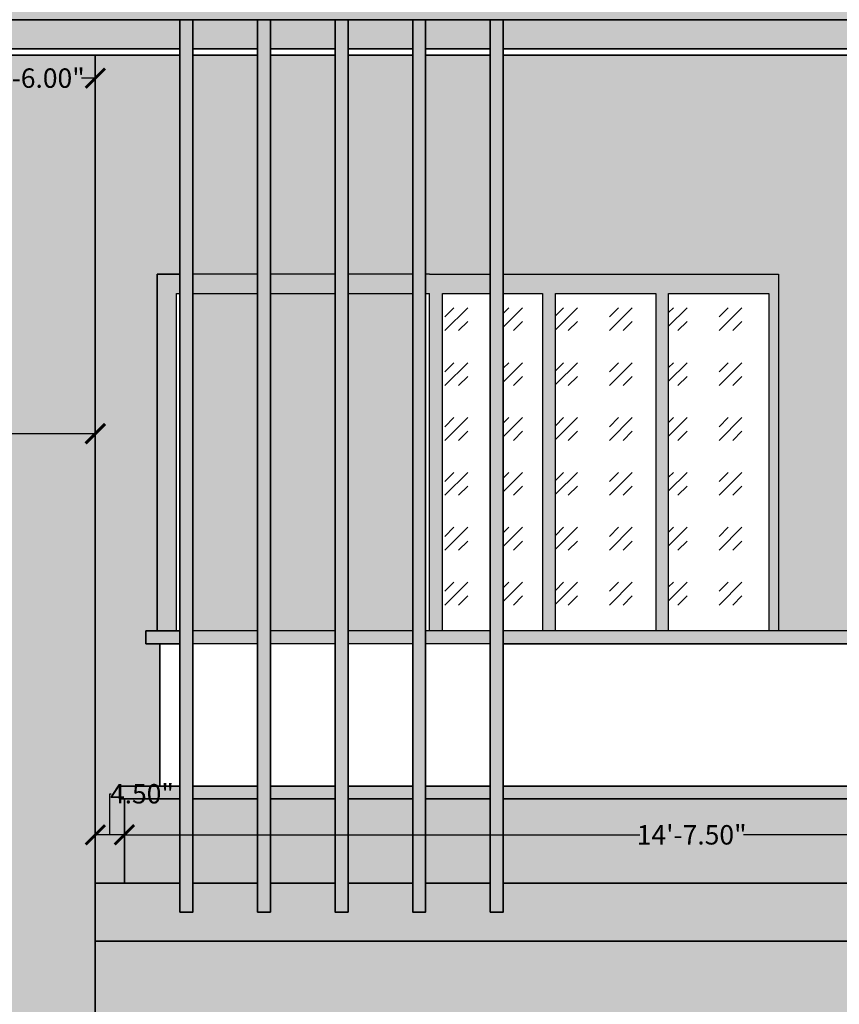
# Model space of a CAD drawing. Units: inches. Extents: x -654 to 390, y -40 to 648.
# Tile 6 of 13: x 104 to 231, y 159 to 311. Entities that reach past the tile are written whole.
import ezdxf

# ---------------------------------------------------------------- set-up
doc = ezdxf.new("R2010")
doc.units = ezdxf.units.IN
doc.header["$PDMODE"] = 3
for name, color, linetype, lineweight in [('A-ANNO-DIMS', 2, 'Continuous', 18), ('A-ELEV', 7, 'Continuous', 35), ('A-ELEV-FILL', 252, 'Continuous', 13), ('A-ELEV-PATT', 8, 'Continuous', 13), ('A-GLAZ', 4, 'Continuous', 25)]:
    doc.layers.add(name, color=color, linetype=linetype, lineweight=lineweight)
doc.styles.get("Standard").update_dxf_attribs({"font": 'arial.ttf'})
doc.dimstyles.get("Standard").update_dxf_attribs({"dimtxt": 3, "dimasz": 3, "dimexe": 0.18, "dimexo": 0.0625, "dimgap": 0.09, "dimtad": 0, "dimtih": 1, "dimtoh": 1, "dimzin": 0, "dimdsep": 46, "dimlunit": 3, "dimtxsty": 'Standard', "dimblk": 'ARCHTICK', "dimcen": 0.09, "dimse1": 1, "dimse2": 1, "dimadec": 0, "dimazin": 0, "dimtfac": 1, "dimtofl": 0, "dimtmove": 0, "dimatfit": 3, "dimfxl": 1, "dimtolj": 1, "dimtzin": 0, "dimarcsym": 0})

# ---------------------------------------------------------------- blocks, each defined once
blk = doc.blocks.new('_ArchTick')
at = {"color": 0, "linetype": 'ByBlock', "const_width": 0.15}
blk.add_lwpolyline([(-0.5, -0.5), (0.5, 0.5)], dxfattribs=at)
blk = doc.blocks.new('*D60')
at = {"layer": 'A-ANNO-DIMS', "color": 0, "lineweight": -2, "transparency": 16777216}
for p, q in [((120.15, 185.09), (199.88, 185.09)), ((295.65, 185.09), (215.91, 185.09))]:
    blk.add_line(p, q, dxfattribs=at)
at = {"layer": 'Defpoints', "color": 0, "transparency": 16777216}
for p in [(120.15, 185.09), (120.15, 185.09), (295.65, 185.09)]:
    blk.add_point(p, dxfattribs=at)
at = {"layer": 'A-ANNO-DIMS', "color": 0, "lineweight": -2, "transparency": 16777216, "xscale": 3, "yscale": 3, "zscale": 3, "rotation": 180}
blk.add_blockref('_ArchTick', (120.15, 185.09), dxfattribs=at)
at = {"layer": 'A-ANNO-DIMS', "color": 0, "lineweight": -2, "transparency": 16777216, "xscale": 3, "yscale": 3, "zscale": 3}
blk.add_blockref('_ArchTick', (295.65, 185.09), dxfattribs=at)
at = {"layer": 'A-ANNO-DIMS', "color": 0, "transparency": 16777216, "insert": (207.9, 185.09), "char_height": 3, "attachment_point": 5}
blk.add_mtext('\\A1;14\'-7.50"', dxfattribs=at)
blk = doc.blocks.new('*D61')
at = {"layer": 'A-ANNO-DIMS', "color": 0, "lineweight": -2, "transparency": 16777216}
for p, q in [((117.9, 185.09), (117.9, 191.44)), ((117.9, 191.44), (118.08, 191.44)), ((120.15, 185.09), (115.65, 185.09))]:
    blk.add_line(p, q, dxfattribs=at)
at = {"layer": 'Defpoints', "color": 0, "transparency": 16777216}
for p in [(115.65, 185.09), (115.65, 185.09), (120.15, 185.09)]:
    blk.add_point(p, dxfattribs=at)
at = {"layer": 'A-ANNO-DIMS', "color": 0, "lineweight": -2, "transparency": 16777216, "xscale": 3, "yscale": 3, "zscale": 3, "rotation": 180}
blk.add_blockref('_ArchTick', (115.65, 185.09), dxfattribs=at)
at = {"layer": 'A-ANNO-DIMS', "color": 0, "lineweight": -2, "transparency": 16777216, "xscale": 3, "yscale": 3, "zscale": 3}
blk.add_blockref('_ArchTick', (120.15, 185.09), dxfattribs=at)
at = {"layer": 'A-ANNO-DIMS', "color": 0, "transparency": 16777216, "insert": (122.86, 191.44), "char_height": 3, "attachment_point": 5}
blk.add_mtext('\\A1;4.50"', dxfattribs=at)
blk = doc.blocks.new('*D69')
at = {"layer": 'A-ANNO-DIMS', "color": 0, "lineweight": -2, "transparency": 16777216}
for p, q in [((57.15, 247.12), (78.18, 247.12)), ((115.65, 247.12), (94.61, 247.12))]:
    blk.add_line(p, q, dxfattribs=at)
at = {"layer": 'Defpoints', "color": 0, "transparency": 16777216}
for p in [(115.65, 247.12), (115.65, 177.63), (57.15, 161.13)]:
    blk.add_point(p, dxfattribs=at)
at = {"layer": 'A-ANNO-DIMS', "color": 0, "lineweight": -2, "transparency": 16777216, "xscale": 3, "yscale": 3, "zscale": 3, "rotation": 180}
blk.add_blockref('_ArchTick', (57.15, 247.12), dxfattribs=at)
at = {"layer": 'A-ANNO-DIMS', "color": 0, "lineweight": -2, "transparency": 16777216, "xscale": 3, "yscale": 3, "zscale": 3}
blk.add_blockref('_ArchTick', (115.65, 247.12), dxfattribs=at)
at = {"layer": 'A-ANNO-DIMS', "color": 0, "transparency": 16777216, "insert": (86.4, 247.12), "char_height": 3, "attachment_point": 5}
blk.add_mtext('\\A1;4\'-10.50"', dxfattribs=at)
blk = doc.blocks.new('*D70')
at = {"layer": 'A-ANNO-DIMS', "color": 0, "lineweight": -2, "transparency": 16777216}
for p, q in [((97.65, 302.1), (99.8, 302.1)), ((115.65, 302.1), (113.5, 302.1))]:
    blk.add_line(p, q, dxfattribs=at)
at = {"layer": 'Defpoints', "color": 0, "transparency": 16777216}
for p in [(97.65, 305.63), (115.65, 305.63), (115.65, 302.1)]:
    blk.add_point(p, dxfattribs=at)
at = {"layer": 'A-ANNO-DIMS', "color": 0, "lineweight": -2, "transparency": 16777216, "xscale": 3, "yscale": 3, "zscale": 3, "rotation": 180}
blk.add_blockref('_ArchTick', (97.65, 302.1), dxfattribs=at)
at = {"layer": 'A-ANNO-DIMS', "color": 0, "lineweight": -2, "transparency": 16777216, "xscale": 3, "yscale": 3, "zscale": 3}
blk.add_blockref('_ArchTick', (115.65, 302.1), dxfattribs=at)
at = {"layer": 'A-ANNO-DIMS', "color": 0, "transparency": 16777216, "insert": (106.65, 302.1), "char_height": 3, "attachment_point": 5}
blk.add_mtext('\\A1;1\'-6.00"', dxfattribs=at)
blk = doc.blocks.new('*D76')
at = {"layer": 'A-ANNO-DIMS', "color": 0, "lineweight": -2, "transparency": 16777216}
for p, q in [((380.75, 611.13), (380.75, 306.76)), ((380.75, -0.87), (380.75, 303.51))]:
    blk.add_line(p, q, dxfattribs=at)
at = {"layer": 'Defpoints', "color": 0, "transparency": 16777216}
for p in [(126.65, 611.13), (380.75, 611.13), (346.65, -0.87)]:
    blk.add_point(p, dxfattribs=at)
at = {"layer": 'A-ANNO-DIMS', "color": 0, "lineweight": -2, "transparency": 16777216, "xscale": 3, "yscale": 3, "zscale": 3}
for p, rotation in [((380.75, 611.13), 90), ((380.75, -0.87), 270)]:
    blk.add_blockref('_ArchTick', p, dxfattribs=dict(at, rotation=rotation))
at = {"layer": 'A-ANNO-DIMS', "color": 0, "transparency": 16777216, "insert": (380.75, 305.13), "char_height": 3, "attachment_point": 5}
blk.add_mtext('\\A1;51\'-0"', dxfattribs=at)
blk = doc.blocks.new('*D92')
at = {"layer": 'A-ANNO-DIMS', "color": 0, "lineweight": -2, "transparency": 16777216}
for p, q in [((115.65, -32.97), (125.23, -32.97)), ((125.23, -32.97), (128.23, -32.97))]:
    blk.add_line(p, q, dxfattribs=at)
at = {"layer": 'Defpoints', "color": 0, "transparency": 16777216}
for p in [(115.65, 305.63), (125.23, 271.79), (125.23, -32.97)]:
    blk.add_point(p, dxfattribs=at)
at = {"layer": 'A-ANNO-DIMS', "color": 0, "lineweight": -2, "transparency": 16777216, "xscale": 3, "yscale": 3, "zscale": 3, "rotation": 180}
blk.add_blockref('_ArchTick', (115.65, -32.97), dxfattribs=at)
at = {"layer": 'A-ANNO-DIMS', "color": 0, "lineweight": -2, "transparency": 16777216, "xscale": 3, "yscale": 3, "zscale": 3}
blk.add_blockref('_ArchTick', (125.23, -32.97), dxfattribs=at)
at = {"layer": 'A-ANNO-DIMS', "color": 0, "transparency": 16777216, "insert": (135.8, -32.97), "char_height": 3, "attachment_point": 5}
blk.add_mtext('\\A1;0\'-9 1/2"', dxfattribs=at)
blk = doc.blocks.new('*D93')
at = {"layer": 'A-ANNO-DIMS', "color": 0, "lineweight": -2, "transparency": 16777216}
for p, q in [((125.23, -32.97), (169.2, -32.97)), ((221.33, -32.97), (177.36, -32.97))]:
    blk.add_line(p, q, dxfattribs=at)
at = {"layer": 'Defpoints', "color": 0, "transparency": 16777216}
for p in [(125.23, 271.79), (221.33, 271.79), (221.33, -32.97)]:
    blk.add_point(p, dxfattribs=at)
at = {"layer": 'A-ANNO-DIMS', "color": 0, "lineweight": -2, "transparency": 16777216, "xscale": 3, "yscale": 3, "zscale": 3, "rotation": 180}
blk.add_blockref('_ArchTick', (125.23, -32.97), dxfattribs=at)
at = {"layer": 'A-ANNO-DIMS', "color": 0, "lineweight": -2, "transparency": 16777216, "xscale": 3, "yscale": 3, "zscale": 3}
blk.add_blockref('_ArchTick', (221.33, -32.97), dxfattribs=at)
at = {"layer": 'A-ANNO-DIMS', "color": 0, "transparency": 16777216, "insert": (173.28, -32.97), "char_height": 3, "attachment_point": 5}
blk.add_mtext('\\A1;8\'-0"', dxfattribs=at)
blk = doc.blocks.new('*D94')
at = {"layer": 'A-ANNO-DIMS', "color": 0, "lineweight": -2, "transparency": 16777216}
for p, q in [((380.75, 271.79), (380.75, 245.8)), ((380.75, 216.63), (380.75, 242.62))]:
    blk.add_line(p, q, dxfattribs=at)
at = {"layer": 'Defpoints', "color": 0, "transparency": 16777216}
for p in [(221.33, 271.79), (244.73, 216.63), (380.75, 216.63)]:
    blk.add_point(p, dxfattribs=at)
at = {"layer": 'A-ANNO-DIMS', "color": 0, "lineweight": -2, "transparency": 16777216, "xscale": 3, "yscale": 3, "zscale": 3}
for p, rotation in [((380.75, 271.79), 90), ((380.75, 216.63), 270)]:
    blk.add_blockref('_ArchTick', p, dxfattribs=dict(at, rotation=rotation))
at = {"layer": 'A-ANNO-DIMS', "color": 0, "transparency": 16777216, "insert": (380.75, 244.21), "char_height": 3, "attachment_point": 5}
blk.add_mtext('\\A1;4\'-7"', dxfattribs=at)
blk = doc.blocks.new('*D97')
at = {"layer": 'A-ANNO-DIMS', "color": 0, "lineweight": -2, "transparency": 16777216}
for p, q in [((128.74, -32.97), (130.81, -32.97)), ((140.74, -32.97), (138.68, -32.97))]:
    blk.add_line(p, q, dxfattribs=at)
at = {"layer": 'Defpoints', "color": 0, "transparency": 16777216}
for p in [(128.74, 173.13), (140.74, 173.13), (140.74, -32.97)]:
    blk.add_point(p, dxfattribs=at)
at = {"layer": 'A-ANNO-DIMS', "color": 0, "lineweight": -2, "transparency": 16777216, "xscale": 3, "yscale": 3, "zscale": 3, "rotation": 180}
blk.add_blockref('_ArchTick', (128.74, -32.97), dxfattribs=at)
at = {"layer": 'A-ANNO-DIMS', "color": 0, "lineweight": -2, "transparency": 16777216, "xscale": 3, "yscale": 3, "zscale": 3}
blk.add_blockref('_ArchTick', (140.74, -32.97), dxfattribs=at)
at = {"layer": 'A-ANNO-DIMS', "color": 0, "transparency": 16777216, "insert": (134.74, -32.97), "char_height": 3, "attachment_point": 5}
blk.add_mtext('\\A1;1\'-0"', dxfattribs=at)
blk = doc.blocks.new('*D98')
at = {"layer": 'A-ANNO-DIMS', "color": 0, "lineweight": -2, "transparency": 16777216}
for p, q in [((128.74, -32.97), (149.6, -32.97)), ((178.74, -32.97), (157.88, -32.97))]:
    blk.add_line(p, q, dxfattribs=at)
at = {"layer": 'Defpoints', "color": 0, "transparency": 16777216}
for p in [(128.74, 173.13), (178.74, 173.13), (178.74, -32.97)]:
    blk.add_point(p, dxfattribs=at)
at = {"layer": 'A-ANNO-DIMS', "color": 0, "lineweight": -2, "transparency": 16777216, "xscale": 3, "yscale": 3, "zscale": 3, "rotation": 180}
blk.add_blockref('_ArchTick', (128.74, -32.97), dxfattribs=at)
at = {"layer": 'A-ANNO-DIMS', "color": 0, "lineweight": -2, "transparency": 16777216, "xscale": 3, "yscale": 3, "zscale": 3}
blk.add_blockref('_ArchTick', (178.74, -32.97), dxfattribs=at)
at = {"layer": 'A-ANNO-DIMS', "color": 0, "transparency": 16777216, "insert": (153.74, -32.97), "char_height": 3, "attachment_point": 5}
blk.add_mtext('\\A1;4\'-2"', dxfattribs=at)
blk = doc.blocks.new('*D99')
at = {"layer": 'A-ANNO-DIMS', "color": 0, "lineweight": -2, "transparency": 16777216}
for p, q in [((380.75, 311.13), (380.75, 243.76)), ((380.75, 173.13), (380.75, 240.51))]:
    blk.add_line(p, q, dxfattribs=at)
at = {"layer": 'Defpoints', "color": 0, "transparency": 16777216}
for p in [(178.74, 311.13), (380.75, 311.13), (178.74, 173.13)]:
    blk.add_point(p, dxfattribs=at)
at = {"layer": 'A-ANNO-DIMS', "color": 0, "lineweight": -2, "transparency": 16777216, "xscale": 3, "yscale": 3, "zscale": 3}
for p, rotation in [((380.75, 311.13), 90), ((380.75, 173.13), 270)]:
    blk.add_blockref('_ArchTick', p, dxfattribs=dict(at, rotation=rotation))
at = {"layer": 'A-ANNO-DIMS', "color": 0, "transparency": 16777216, "insert": (380.75, 242.13), "char_height": 3, "attachment_point": 5}
blk.add_mtext('\\A1;11\'-6"', dxfattribs=at)
blk = doc.blocks.new('*D100')
at = {"layer": 'A-ANNO-DIMS', "color": 0, "lineweight": -2, "transparency": 16777216}
for p, q in [((145.65, -32.97), (157.49, -32.97)), ((179.88, -32.97), (168.03, -32.97))]:
    blk.add_line(p, q, dxfattribs=at)
at = {"layer": 'Defpoints', "color": 0, "transparency": 16777216}
for p in [(145.65, 355.63), (179.88, 355.63), (179.88, -32.97)]:
    blk.add_point(p, dxfattribs=at)
at = {"layer": 'A-ANNO-DIMS', "color": 0, "lineweight": -2, "transparency": 16777216, "xscale": 3, "yscale": 3, "zscale": 3, "rotation": 180}
blk.add_blockref('_ArchTick', (145.65, -32.97), dxfattribs=at)
at = {"layer": 'A-ANNO-DIMS', "color": 0, "lineweight": -2, "transparency": 16777216, "xscale": 3, "yscale": 3, "zscale": 3}
blk.add_blockref('_ArchTick', (179.88, -32.97), dxfattribs=at)
at = {"layer": 'A-ANNO-DIMS', "color": 0, "transparency": 16777216, "insert": (162.76, -32.97), "char_height": 3, "attachment_point": 5}
blk.add_mtext('\\A1;2\'-10"', dxfattribs=at)
blk = doc.blocks.new('*D102')
at = {"layer": 'A-ANNO-DIMS', "color": 0, "lineweight": -2, "transparency": 16777216}
for p, q in [((179.88, -32.97), (205.8, -32.97)), ((239.87, -32.97), (213.95, -32.97))]:
    blk.add_line(p, q, dxfattribs=at)
at = {"layer": 'Defpoints', "color": 0, "transparency": 16777216}
for p in [(179.88, 355.63), (239.87, 355.63), (239.87, -32.97)]:
    blk.add_point(p, dxfattribs=at)
at = {"layer": 'A-ANNO-DIMS', "color": 0, "lineweight": -2, "transparency": 16777216, "xscale": 3, "yscale": 3, "zscale": 3, "rotation": 180}
blk.add_blockref('_ArchTick', (179.88, -32.97), dxfattribs=at)
at = {"layer": 'A-ANNO-DIMS', "color": 0, "lineweight": -2, "transparency": 16777216, "xscale": 3, "yscale": 3, "zscale": 3}
blk.add_blockref('_ArchTick', (239.87, -32.97), dxfattribs=at)
at = {"layer": 'A-ANNO-DIMS', "color": 0, "transparency": 16777216, "insert": (209.87, -32.97), "char_height": 3, "attachment_point": 5}
blk.add_mtext('\\A1;5\'-0"', dxfattribs=at)

msp = doc.modelspace()

# ---------------------------------------------------------------- hatches: boundary and pattern name
at = {"layer": 'A-ELEV-FILL'}
h = msp.add_hatch(color=256, dxfattribs=at)
h.dxf.hatch_style = 1
h.paths.add_polyline_path([(115.646, 305.634), (97.646, 305.634), (97.646, 306.634), (98.293, 306.634), (98.293, 315.634), (97.646, 315.634), (97.646, 316.634), (100.646, 316.634), (100.646, 442.634), (-1.354, 442.634), (-1.354, 125.134), (115.646, 125.134)])
h.paths.add_polyline_path([(57.146, 161.134), (12.146, 161.134), (12.146, 413.134), (57.146, 413.134)], flags=16)
h.paths.add_polyline_path([(52.646, 165.634), (16.646, 165.634), (16.646, 408.634), (52.646, 408.634)], flags=0)
h.paths.add_polyline_path([(52.146, 166.134), (17.146, 166.134), (17.146, 408.134), (52.146, 408.134)], flags=0)
h.paths.add_polyline_path([(124.646, 581.134), (-1.354, 581.134), (-1.354, 497.134), (8.646, 497.134), (8.646, 494.634), (12.146, 494.634), (12.146, 546.634), (57.146, 546.634), (57.146, 494.634), (124.646, 494.634)])
h.paths.add_polyline_path([(124.646, 609.134), (-1.354, 609.134), (-1.354, 590.134), (124.646, 590.134)])
h = msp.add_hatch(color=256, dxfattribs=at)
h.dxf.hatch_style = 1
h.paths.add_polyline_path([(161.035, 590.134), (-1.354, 590.134), (-1.354, 581.134), (161.035, 581.134)])
h.paths.add_polyline_path([(346.646, 453.634), (-1.354, 453.634), (-1.354, 444.634), (337.646, 444.634), (337.646, 177.634), (178.742, 177.634), (178.742, 173.134), (176.742, 173.134), (176.742, 177.634), (166.742, 177.634), (166.742, 173.134), (164.742, 173.134), (164.742, 177.634), (154.742, 177.634), (154.742, 173.134), (152.742, 173.134), (152.742, 177.634), (142.742, 177.634), (142.742, 173.134), (140.742, 173.134), (140.742, 177.634), (130.742, 177.634), (130.742, 173.134), (128.742, 173.134), (128.742, 177.634), (115.646, 177.634), (115.646, 168.634), (346.646, 168.634), (346.646, 173.134)])
h.paths.add_polyline_path([(7.646, 87.642), (-1.354, 87.642), (-1.354, 17.134), (7.646, 17.134)])
h.paths.add_polyline_path([(16.396, 116.134), (60.646, 116.134), (60.646, 83.134), (62.646, 83.134), (113.646, 83.134), (115.646, 83.134), (115.646, 125.134), (7.646, 125.134), (7.646, 89.642), (8.146, 89.642), (8.146, 87.642), (7.646, 87.642), (7.646, 83.134), (9.646, 83.134), (16.396, 83.134)])
h = msp.add_hatch(color=256, dxfattribs=at)
h.dxf.hatch_style = 1
h.paths.add_polyline_path([(346.646, 587.634), (161.035, 587.634), (161.035, 583.634), (342.646, 583.634), (342.646, 497.134), (346.646, 497.134), (346.646, 583.634)])
h.paths.add_polyline_path([(295.646, 315.634), (98.293, 315.634), (98.293, 311.134), (295.646, 311.134)])
h.paths.add_polyline_path([(128.742, 311.134), (98.293, 311.134), (98.293, 306.634), (128.742, 306.634)])
h.paths.add_polyline_path([(140.742, 311.134), (130.742, 311.134), (130.742, 306.634), (140.742, 306.634)])
h.paths.add_polyline_path([(152.742, 311.134), (142.742, 311.134), (142.742, 306.634), (152.742, 306.634)])
h.paths.add_polyline_path([(164.742, 311.134), (154.742, 311.134), (154.742, 306.634), (164.742, 306.634)])
h.paths.add_polyline_path([(176.742, 311.134), (166.742, 311.134), (166.742, 306.634), (176.742, 306.634)])
h.paths.add_polyline_path([(295.646, 311.134), (178.742, 311.134), (178.742, 306.634), (295.646, 306.634)])
h.paths.add_polyline_path([(303.818, 315.634), (295.646, 315.634), (295.646, 311.134), (303.818, 311.134)])
h.paths.add_polyline_path([(303.818, 311.134), (295.646, 311.134), (295.646, 306.634), (303.818, 306.634)])
h = msp.add_hatch(color=256, dxfattribs=at)
h.dxf.hatch_style = 1
h.paths.add_polyline_path([(295.646, 190.634), (178.742, 190.634), (178.742, 177.634), (295.646, 177.634)])
h.paths.add_polyline_path([(176.742, 190.634), (166.742, 190.634), (166.742, 177.634), (176.742, 177.634)])
h.paths.add_polyline_path([(164.742, 190.634), (154.742, 190.634), (154.742, 177.634), (164.742, 177.634)])
h.paths.add_polyline_path([(152.742, 190.634), (142.742, 190.634), (142.742, 177.634), (152.742, 177.634)])
h.paths.add_polyline_path([(140.742, 190.634), (130.742, 190.634), (130.742, 177.634), (140.742, 177.634)])
h.paths.add_polyline_path([(128.742, 190.634), (120.146, 190.634), (120.146, 177.634), (128.742, 177.634)])
h.paths.add_polyline_path([(295.646, 329.634), (145.646, 329.634), (145.646, 442.634), (100.646, 442.634), (100.646, 316.634), (295.646, 316.634)])
h.paths.add_polyline_path([(138.646, 359.634), (107.646, 359.634), (107.646, 438.634), (138.646, 438.634)], flags=16)
h.paths.add_polyline_path([(136.646, 361.634), (109.646, 361.634), (109.646, 436.634), (136.646, 436.634)], flags=0)
h.paths.add_polyline_path([(184.646, 466.634), (7.646, 466.634), (7.646, 453.634), (184.646, 453.634)])
h.paths.add_polyline_path([(184.646, 494.634), (7.646, 494.634), (7.646, 492.634), (184.646, 492.634)])
h.paths.add_polyline_path([(10.336, 492.634), (9.336, 492.634), (9.336, 468.634), (10.336, 468.634)])
h.paths.add_polyline_path([(17.352, 492.634), (16.352, 492.634), (16.352, 468.634), (17.352, 468.634)])
h.paths.add_polyline_path([(24.368, 492.634), (23.368, 492.634), (23.368, 468.634), (24.368, 468.634)])
h.paths.add_polyline_path([(31.384, 492.634), (30.384, 492.634), (30.384, 468.634), (31.384, 468.634)])
h.paths.add_polyline_path([(38.4, 492.634), (37.4, 492.634), (37.4, 468.634), (38.4, 468.634)])
h.paths.add_polyline_path([(45.416, 492.634), (44.416, 492.634), (44.416, 468.634), (45.416, 468.634)])
h.paths.add_polyline_path([(52.432, 492.634), (51.432, 492.634), (51.432, 468.634), (52.432, 468.634)])
h.paths.add_polyline_path([(59.448, 492.634), (58.448, 492.634), (58.448, 468.634), (59.448, 468.634)])
h.paths.add_polyline_path([(66.464, 492.634), (65.464, 492.634), (65.464, 468.634), (66.464, 468.634)])
h.paths.add_polyline_path([(73.48, 492.634), (72.48, 492.634), (72.48, 468.634), (73.48, 468.634)])
h.paths.add_polyline_path([(80.496, 492.634), (79.496, 492.634), (79.496, 468.634), (80.496, 468.634)])
h.paths.add_polyline_path([(87.512, 492.634), (86.512, 492.634), (86.512, 468.634), (87.512, 468.634)])
h.paths.add_polyline_path([(94.528, 492.634), (93.528, 492.634), (93.528, 468.634), (94.528, 468.634)])
h.paths.add_polyline_path([(101.544, 492.634), (100.544, 492.634), (100.544, 468.634), (101.544, 468.634)])
h.paths.add_polyline_path([(108.559, 492.634), (107.559, 492.634), (107.559, 468.634), (108.559, 468.634)])
h.paths.add_polyline_path([(115.575, 492.634), (114.575, 492.634), (114.575, 468.634), (115.575, 468.634)])
h.paths.add_polyline_path([(122.591, 492.634), (121.591, 492.634), (121.591, 468.634), (122.591, 468.634)])
h.paths.add_polyline_path([(129.607, 492.634), (128.607, 492.634), (128.607, 468.634), (129.607, 468.634)])
h.paths.add_polyline_path([(136.623, 492.634), (135.623, 492.634), (135.623, 468.634), (136.623, 468.634)])
h.paths.add_polyline_path([(143.639, 492.634), (142.639, 492.634), (142.639, 468.634), (143.639, 468.634)])
h.paths.add_polyline_path([(150.655, 492.634), (149.655, 492.634), (149.655, 468.634), (150.655, 468.634)])
h.paths.add_polyline_path([(157.671, 492.634), (156.671, 492.634), (156.671, 468.634), (157.671, 468.634)])
h.paths.add_polyline_path([(164.687, 492.634), (163.687, 492.634), (163.687, 468.634), (164.687, 468.634)])
h.paths.add_polyline_path([(171.703, 492.634), (170.703, 492.634), (170.703, 468.634), (171.703, 468.634)])
h.paths.add_polyline_path([(178.719, 492.634), (177.719, 492.634), (177.719, 468.634), (178.719, 468.634)])
h = msp.add_hatch(color=256, dxfattribs=at)
h.dxf.hatch_style = 1
h.paths.add_polyline_path([(138.646, 438.634), (107.646, 438.634), (107.646, 359.634), (138.646, 359.634)])
h.paths.add_polyline_path([(136.646, 436.634), (136.646, 361.634), (109.646, 361.634), (109.646, 436.634)], flags=16)
h.paths.add_polyline_path([(179.877, 410.786), (145.646, 410.786), (145.646, 407.786), (153.285, 407.786), (153.285, 357.634), (145.646, 357.634), (145.646, 355.634), (179.877, 355.634)])
h.paths.add_polyline_path([(178.123, 407.786), (178.123, 357.634), (155.286, 357.634), (155.286, 407.786)], flags=16)
h.paths.add_polyline_path([(291.141, 410.786), (239.871, 410.786), (239.871, 355.634), (241.996, 355.634), (241.996, 407.786), (269.317, 407.786), (269.317, 355.634), (271.318, 355.634), (271.318, 407.786), (289.369, 407.786), (289.369, 355.634), (291.141, 355.634)])
h.paths.add_polyline_path([(128.225, 268.786), (128.742, 268.786), (128.742, 271.786), (125.225, 271.786), (125.225, 216.634), (128.225, 216.634)])
h.paths.add_polyline_path([(140.742, 271.786), (130.742, 271.786), (130.742, 268.786), (140.742, 268.786)])
h.paths.add_polyline_path([(152.742, 271.786), (142.742, 271.786), (142.742, 268.786), (152.742, 268.786)])
h.paths.add_polyline_path([(164.742, 271.786), (154.742, 271.786), (154.742, 268.786), (164.742, 268.786)])
h.paths.add_polyline_path([(176.742, 271.786), (167.328, 271.786), (166.742, 271.786), (166.742, 268.786), (167.328, 268.786), (167.328, 216.634), (169.328, 216.634), (169.328, 268.786), (176.742, 268.786)])
h.paths.add_polyline_path([(221.328, 271.786), (178.742, 271.786), (178.742, 268.786), (184.828, 268.786), (184.828, 216.634), (186.829, 216.634), (186.829, 268.786), (202.329, 268.786), (202.329, 216.634), (204.325, 216.634), (204.325, 268.786), (219.825, 268.786), (219.825, 216.634), (221.328, 216.634)])
h.paths.add_polyline_path([(295.646, 271.786), (244.726, 271.786), (244.726, 216.634), (246.481, 216.634), (246.481, 268.786), (269.317, 268.786), (269.317, 216.634), (271.318, 216.634), (271.318, 268.786), (286.818, 268.786), (286.818, 216.634), (288.814, 216.634), (288.814, 268.786), (295.646, 268.786)])
h.paths.add_polyline_path([(295.646, 216.634), (178.742, 216.634), (178.742, 214.634), (295.646, 214.634)])
h.paths.add_polyline_path([(128.742, 216.634), (123.485, 216.634), (123.485, 214.634), (128.742, 214.634)])
h.paths.add_polyline_path([(140.742, 216.634), (130.742, 216.634), (130.742, 214.634), (140.742, 214.634)])
h.paths.add_polyline_path([(152.742, 216.634), (142.742, 216.634), (142.742, 214.634), (152.742, 214.634)])
h.paths.add_polyline_path([(164.742, 216.634), (154.742, 216.634), (154.742, 214.634), (164.742, 214.634)])
h.paths.add_polyline_path([(176.742, 216.634), (166.742, 216.634), (166.742, 214.634), (176.742, 214.634)])
h.paths.add_polyline_path([(128.742, 192.634), (119.386, 192.634), (119.386, 190.634), (128.742, 190.634)])
h.paths.add_polyline_path([(140.742, 192.634), (130.742, 192.634), (130.742, 190.634), (140.742, 190.634)])
h.paths.add_polyline_path([(152.742, 192.634), (142.742, 192.634), (142.742, 190.634), (152.742, 190.634)])
h.paths.add_polyline_path([(164.742, 192.634), (154.742, 192.634), (154.742, 190.634), (164.742, 190.634)])
h.paths.add_polyline_path([(176.742, 192.634), (166.742, 192.634), (166.742, 190.634), (176.742, 190.634)])
h.paths.add_polyline_path([(295.646, 192.634), (178.742, 192.634), (178.742, 190.634), (295.646, 190.634)])
h.paths.add_polyline_path([(189.362, 137.63), (135.362, 137.63), (135.362, 71.63), (189.362, 71.63)])
h.paths.add_polyline_path([(154.862, 134.63), (170.362, 134.63), (170.362, 74.63), (154.862, 74.63)], flags=16)
h.paths.add_polyline_path([(152.862, 134.63), (152.862, 74.63), (137.362, 74.63), (137.362, 134.63)], flags=16)
h.paths.add_polyline_path([(172.358, 134.63), (187.858, 134.63), (187.858, 74.63), (172.358, 74.63)], flags=16)
h.paths.add_polyline_path([(113.646, 83.134), (62.646, 83.134), (62.646, 17.134), (113.646, 17.134)])
h.paths.add_polyline_path([(96.484, 80.08), (109.984, 80.08), (109.984, 20.08), (96.484, 20.08)], flags=16)
h.paths.add_polyline_path([(93.843, 80.08), (93.843, 20.08), (80.343, 20.08), (80.343, 80.08)], flags=16)
h.paths.add_polyline_path([(78.051, 80.08), (78.051, 20.08), (64.551, 20.08), (64.551, 80.08)], flags=16)
h.paths.add_polyline_path([(60.646, 83.134), (9.646, 83.134), (9.646, 17.134), (60.646, 17.134)])
h.paths.add_polyline_path([(58.197, 80.08), (58.197, 20.08), (44.697, 20.08), (44.697, 80.08)], flags=16)
h.paths.add_polyline_path([(41.55, 80.08), (41.55, 20.08), (28.05, 20.08), (28.05, 80.08)], flags=16)
h.paths.add_polyline_path([(25.146, 80.08), (25.146, 20.08), (11.646, 20.08), (11.646, 80.08)], flags=16)
h.paths.add_polyline_path([(9.646, 83.134), (7.646, 83.134), (7.646, 73.776), (9.646, 73.776)])
h.paths.add_polyline_path([(9.646, 65.663), (7.646, 65.663), (7.646, 36.041), (9.646, 36.041)])
h.paths.add_polyline_path([(9.646, 27.928), (7.646, 27.928), (7.646, 17.134), (9.646, 17.134)])
h.paths.add_polyline_path([(115.646, 83.134), (113.646, 83.134), (113.646, 73.776), (115.646, 73.776)])
h.paths.add_polyline_path([(115.646, 65.663), (113.646, 65.663), (113.646, 35.502), (115.646, 35.502)])
h.paths.add_polyline_path([(115.646, 27.389), (113.646, 27.389), (113.646, 17.134), (115.646, 17.134)])
h.paths.add_polyline_path([(8.146, 89.642), (-1.854, 89.642), (-1.854, 87.642), (8.146, 87.642)])
h.paths.add_polyline_path([(245.646, 156.634), (243.646, 156.634), (243.646, 17.134), (245.646, 17.134)])
h.paths.add_polyline_path([(339.646, 156.634), (337.646, 156.634), (337.646, 17.134), (339.646, 17.134)])
h = msp.add_hatch(color=256, dxfattribs=at)
h.dxf.hatch_style = 1
h.paths.add_polyline_path([(269.317, 268.786), (246.481, 268.786), (246.481, 216.634), (269.317, 216.634)])
h.paths.add_polyline_path([(269.317, 407.786), (241.996, 407.786), (241.996, 355.634), (269.317, 355.634)])
h.paths.add_polyline_path([(140.742, 268.786), (130.742, 268.786), (130.742, 216.634), (140.742, 216.634)])
h.paths.add_polyline_path([(152.742, 268.786), (142.742, 268.786), (142.742, 216.634), (152.742, 216.634)])
h.paths.add_polyline_path([(164.742, 268.786), (154.742, 268.786), (154.742, 216.634), (164.742, 216.634)])
h = msp.add_hatch(color=256, dxfattribs=at)
h.dxf.hatch_style = 1
h.paths.add_polyline_path([(130.742, 311.134), (128.742, 311.134), (128.742, 173.134), (130.742, 173.134)])
h.paths.add_polyline_path([(142.742, 311.134), (140.742, 311.134), (140.742, 173.134), (142.742, 173.134)])
h.paths.add_polyline_path([(154.742, 311.134), (152.742, 311.134), (152.742, 173.134), (154.742, 173.134)])
h.paths.add_polyline_path([(166.742, 311.134), (164.742, 311.134), (164.742, 173.134), (166.742, 173.134)])
h.paths.add_polyline_path([(178.742, 311.134), (176.742, 311.134), (176.742, 173.134), (178.742, 173.134)])
h = msp.add_hatch(color=256, dxfattribs=at)
h.dxf.hatch_style = 1
h.paths.add_polyline_path([(295.646, 305.634), (178.742, 305.634), (178.742, 271.786), (221.328, 271.786), (221.328, 216.634), (244.726, 216.634), (244.726, 271.786), (295.646, 271.786)])
h.paths.add_polyline_path([(140.742, 305.634), (130.742, 305.634), (130.742, 271.786), (140.742, 271.786)])
h.paths.add_polyline_path([(152.742, 305.634), (142.742, 305.634), (142.742, 271.786), (152.742, 271.786)])
h.paths.add_polyline_path([(164.742, 305.634), (154.742, 305.634), (154.742, 271.786), (164.742, 271.786)])
h.paths.add_polyline_path([(176.742, 305.634), (166.742, 305.634), (166.742, 271.786), (167.328, 271.786), (176.742, 271.786)])
h.paths.add_polyline_path([(128.742, 305.634), (115.646, 305.634), (115.646, 177.634), (120.146, 177.634), (120.146, 190.634), (119.386, 190.634), (119.386, 192.634), (125.646, 192.634), (125.646, 214.634), (123.485, 214.634), (123.485, 216.634), (125.225, 216.634), (125.225, 271.786), (128.742, 271.786)])
h = msp.add_hatch(color=256, dxfattribs=at)
h.dxf.hatch_style = 1
h.paths.add_polyline_path([(243.646, 156.634), (243.146, 156.634), (243.146, 166.634), (340.146, 166.634), (340.146, 156.634), (339.646, 156.634), (339.646, 35.134), (346.646, 35.134), (346.646, 168.634), (115.646, 168.634), (115.646, 17.134), (118.646, 17.134), (118.646, -0.866), (226.646, -0.866), (226.646, 17.134), (243.646, 17.134)])
h.paths.add_polyline_path([(189.362, 71.63), (135.362, 71.63), (135.362, 137.63), (189.362, 137.63)], flags=16)
h.paths.add_polyline_path([(187.858, 74.63), (172.358, 74.63), (172.358, 134.63), (187.858, 134.63)], flags=0)
h.paths.add_polyline_path([(170.362, 74.63), (154.862, 74.63), (154.862, 134.63), (170.362, 134.63)], flags=0)
h.paths.add_polyline_path([(152.862, 74.63), (137.362, 74.63), (137.362, 134.63), (152.862, 134.63)], flags=0)
h.paths.add_polyline_path([(346.646, 35.134), (339.646, 35.134), (339.646, 17.134), (346.646, 17.134)], flags=17)
at = {"layer": 'A-ELEV-PATT'}
h = msp.add_hatch(dxfattribs=at)
h.set_pattern_fill('GOST_GLASS', color=256)
h.paths.add_polyline_path([(289.369, 407.786), (271.318, 407.786), (271.318, 355.634), (289.369, 355.634)])
h.paths.add_polyline_path([(178.123, 407.786), (155.286, 407.786), (155.286, 357.634), (178.123, 357.634)])
h.paths.add_polyline_path([(153.285, 407.786), (145.646, 407.786), (145.646, 357.634), (153.285, 357.634)])
h.paths.add_polyline_path([(184.828, 268.786), (178.742, 268.786), (178.742, 216.634), (184.828, 216.634)])
h.paths.add_polyline_path([(176.742, 268.786), (169.328, 268.786), (169.328, 216.634), (176.742, 216.634)])
h.paths.add_polyline_path([(202.329, 268.786), (186.829, 268.786), (186.829, 216.634), (202.329, 216.634)])
h.paths.add_polyline_path([(219.825, 268.786), (204.325, 268.786), (204.325, 216.634), (219.825, 216.634)])
h.paths.add_polyline_path([(286.818, 268.786), (271.318, 268.786), (271.318, 216.634), (286.818, 216.634)])
h.paths.add_polyline_path([(295.646, 268.786), (288.814, 268.786), (288.814, 216.634), (295.646, 216.634)])

# ---------------------------------------------------------------- linework, layer by layer
at = {"layer": 'A-ELEV'}
for p, q in [((98.293, 311.134), (303.818, 311.134)), ((97.646, 306.634), (128.742, 306.634)), ((130.742, 306.634), (140.742, 306.634)), ((142.742, 306.634), (152.742, 306.634)), ((154.742, 306.634), (164.742, 306.634)), ((166.742, 306.634), (176.742, 306.634)), ((178.742, 306.634), (304.646, 306.634)), ((97.646, 305.634), (128.742, 305.634)), ((115.646, 17.134), (115.646, 305.634)), ((130.742, 305.634), (140.742, 305.634)), ((142.742, 305.634), (152.742, 305.634)), ((154.742, 305.634), (164.742, 305.634)), ((166.742, 305.634), (176.742, 305.634)), ((178.742, 305.634), (304.646, 305.634)), ((125.225, 216.634), (125.225, 271.786)), ((128.742, 271.786), (125.225, 271.786)), ((123.485, 214.634), (123.485, 216.634)), ((128.742, 216.634), (123.485, 216.634)), ((128.742, 214.634), (123.485, 214.634)), ((125.646, 192.634), (125.646, 214.634)), ((295.646, 214.634), (178.742, 214.634)), ((119.386, 190.634), (119.386, 192.634)), ((128.742, 192.634), (119.386, 192.634)), ((140.742, 192.634), (130.742, 192.634)), ((152.742, 192.634), (142.742, 192.634)), ((164.742, 192.634), (154.742, 192.634)), ((176.742, 192.634), (166.742, 192.634)), ((295.646, 192.634), (178.742, 192.634)), ((128.742, 190.634), (119.386, 190.634)), ((120.146, 177.634), (120.146, 190.634)), ((140.742, 190.634), (130.742, 190.634)), ((152.742, 190.634), (142.742, 190.634)), ((164.742, 190.634), (154.742, 190.634)), ((176.742, 190.634), (166.742, 190.634)), ((295.646, 190.634), (178.742, 190.634)), ((115.646, 177.634), (128.742, 177.634)), ((130.742, 177.634), (140.742, 177.634)), ((142.742, 177.634), (152.742, 177.634)), ((154.742, 177.634), (164.742, 177.634)), ((166.742, 177.634), (176.742, 177.634)), ((178.742, 177.634), (337.646, 177.634)), ((115.646, 168.634), (346.646, 168.634))]:
    msp.add_line(p, q, dxfattribs=at)
for points in [[(128.742, 311.134), (130.742, 311.134), (130.742, 173.134), (128.742, 173.134)], [(140.742, 311.134), (142.742, 311.134), (142.742, 173.134), (140.742, 173.134)], [(152.742, 311.134), (154.742, 311.134), (154.742, 173.134), (152.742, 173.134)], [(164.742, 311.134), (166.742, 311.134), (166.742, 173.134), (164.742, 173.134)], [(176.742, 311.134), (178.742, 311.134), (178.742, 173.134), (176.742, 173.134)]]:
    msp.add_lwpolyline(points, close=True, dxfattribs=at)
at = {"layer": 'A-GLAZ'}
for p, q in [((140.742, 271.786), (130.742, 271.786)), ((152.742, 271.786), (142.742, 271.786)), ((164.742, 271.786), (154.742, 271.786)), ((167.328, 271.786), (166.742, 271.786)), ((128.225, 216.634), (128.225, 268.786)), ((128.225, 268.786), (128.742, 268.786)), ((130.742, 268.786), (140.742, 268.786)), ((142.742, 268.786), (152.742, 268.786)), ((154.742, 268.786), (164.742, 268.786)), ((166.742, 268.786), (167.328, 268.786)), ((140.742, 216.634), (130.742, 216.634)), ((152.742, 216.634), (142.742, 216.634)), ((164.742, 216.634), (154.742, 216.634)), ((176.742, 216.634), (166.742, 216.634)), ((295.646, 216.634), (178.742, 216.634)), ((140.742, 214.634), (130.742, 214.634)), ((152.742, 214.634), (142.742, 214.634)), ((164.742, 214.634), (154.742, 214.634)), ((176.742, 214.634), (166.742, 214.634))]:
    msp.add_line(p, q, dxfattribs=at)
for points in [[(167.328, 271.786), (176.742, 271.786)], [(178.742, 271.786), (221.328, 271.786), (221.328, 216.634)], [(167.328, 216.634), (167.328, 268.786)], [(169.328, 216.634), (169.328, 268.786), (176.742, 268.786)], [(178.742, 268.786), (184.828, 268.786), (184.828, 216.634)], [(186.829, 216.634), (186.829, 268.786), (202.329, 268.786), (202.329, 216.634)], [(204.325, 216.634), (204.325, 268.786), (219.825, 268.786), (219.825, 216.634)]]:
    msp.add_lwpolyline(points, dxfattribs=at)

# ---------------------------------------------------------------- dimensions: what is measured, and where the dimension line sits
at = {"layer": 'A-ANNO-DIMS'}
for base, p1, p2, picture, middle in [((380.746, 611.134), (346.646, -0.866), (126.646, 611.134), '*D76', (380.746, 305.134)), ((380.746, 311.134), (178.742, 173.134), (178.742, 311.134), '*D99', (380.746, 242.134)), ((380.746, 216.634), (221.328, 271.786), (244.726, 216.634), '*D94', (380.746, 244.21))]:
    dim = msp.add_linear_dim(base=base, p1=p1, p2=p2, angle=90, dimstyle='Standard', override={"dimdec": 1, "dimlfac": 1, "dimrnd": 0, "dimzin": 1, "dimdsep": 46, "dimlunit": 4, "dimfrac": 2}, dxfattribs=at)
    dim.commit()
    dim.dimension.update_dxf_attribs({"geometry": picture, "text_midpoint": middle})
for base, p1, p2, override, picture, middle in [((179.877, -32.966), (145.646, 355.634), (179.877, 355.634), {"dimdec": 1, "dimlfac": 1, "dimrnd": 0, "dimzin": 1, "dimdsep": 46, "dimlunit": 4, "dimfrac": 2}, '*D100', (162.762, -32.966)), ((239.871, -32.966), (179.877, 355.634), (239.871, 355.634), {"dimdec": 1, "dimlfac": 1, "dimrnd": 0, "dimzin": 1, "dimdsep": 46, "dimlunit": 4, "dimfrac": 2}, '*D102', (209.874, -32.966)), ((115.646, 302.096), (97.646, 305.634), (115.646, 305.634), {"dimclrd": 0, "dimclre": 0, "dimclrt": 0}, '*D70', (106.646, 302.096)), ((125.225, -32.966), (115.646, 305.634), (125.225, 271.786), {"dimdec": 1, "dimlfac": 1, "dimrnd": 0, "dimzin": 1, "dimdsep": 46, "dimlunit": 4, "dimfrac": 2}, '*D92', (135.798, -32.966)), ((221.328, -32.966), (125.225, 271.786), (221.328, 271.786), {"dimdec": 1, "dimlfac": 1, "dimrnd": 0, "dimzin": 1, "dimdsep": 46, "dimlunit": 4, "dimfrac": 2}, '*D93', (173.277, -32.966)), ((115.646, 247.118), (57.146, 161.134), (115.646, 177.634), {"dimclrd": 0, "dimclre": 0, "dimclrt": 0}, '*D69', (86.396, 247.118)), ((115.646, 185.092), (120.146, 185.092), (115.646, 185.092), {"dimclrd": 0, "dimclre": 0, "dimclrt": 0, "dimtmove": 1}, '*D61', (118.166, 191.443)), ((120.146, 185.092), (295.646, 185.092), (120.146, 185.092), {"dimclrd": 0, "dimclre": 0, "dimclrt": 0, "dimtmove": 1}, '*D60', (207.896, 185.092)), ((140.742, -32.966), (128.742, 173.134), (140.742, 173.134), {"dimdec": 1, "dimlfac": 1, "dimrnd": 0, "dimzin": 1, "dimdsep": 46, "dimlunit": 4, "dimfrac": 2}, '*D97', (134.742, -32.966)), ((178.742, -32.966), (128.742, 173.134), (178.742, 173.134), {"dimdec": 1, "dimlfac": 1, "dimrnd": 0, "dimzin": 1, "dimdsep": 46, "dimlunit": 4, "dimfrac": 2}, '*D98', (153.742, -32.966))]:
    dim = msp.add_linear_dim(base=base, p1=p1, p2=p2, dimstyle='Standard', override=override, dxfattribs=at)
    dim.commit()
    dim.dimension.update_dxf_attribs({"geometry": picture, "text_midpoint": middle})

doc.saveas('drawing.dxf')
